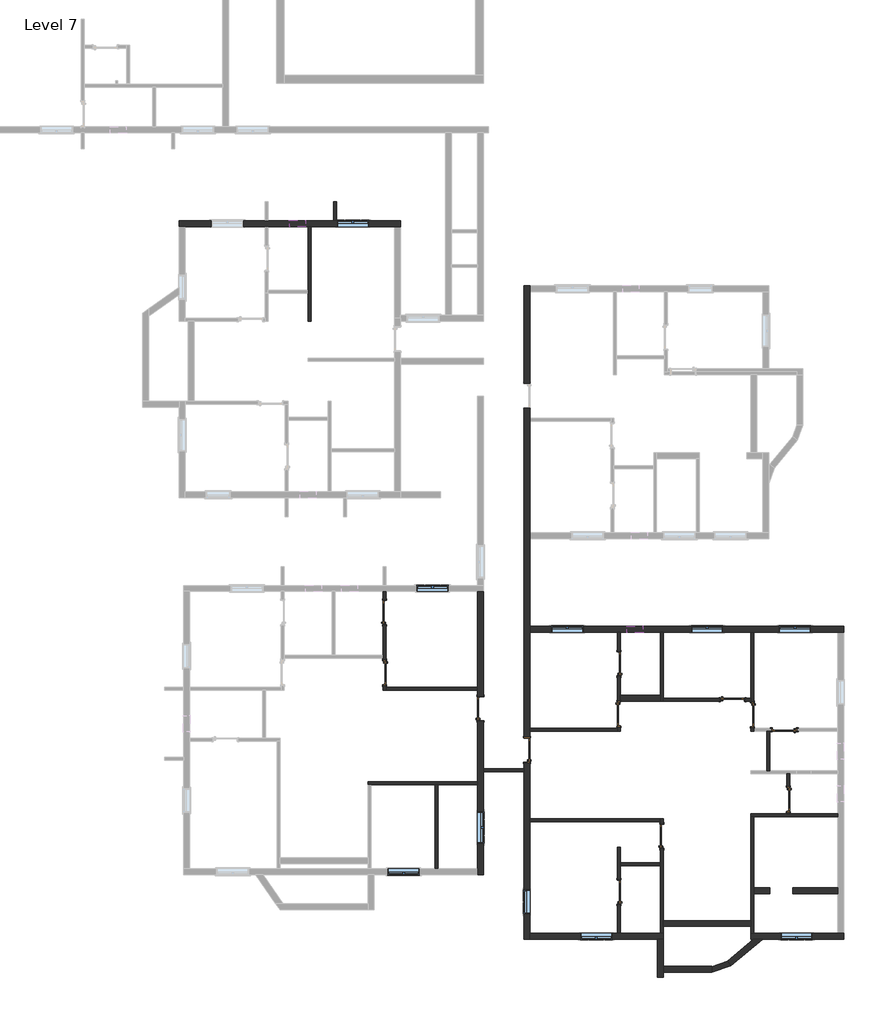
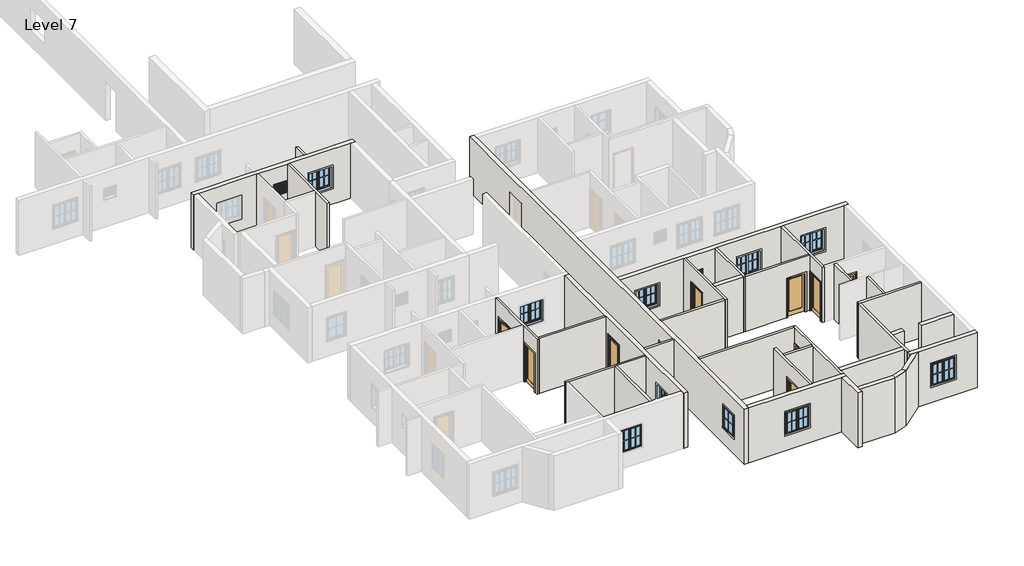
# One storey, part 2 of 7: 34 walls, 12 doors, 12 windows.
"""IFC4 building model written with IfcOpenShell, lengths in millimetres."""

from ifc_helpers import new_model, si_unit, frame, origin, place, context, project, spatial, polyline, circle_curve, outline, extrude, faceted_brep, transform, mapped, element, save
from ifc_brep_helpers import plane_surface, cylinder_surface, revolved_surface, advanced_brep
from components import door_3c6ab76a, door_a3feeac7, door_3b97b8e7, door_868ee8a9, window_272f20d6, window_casement_double_4_x_4_af3140d2, window_f2d8fef0

model = new_model("IFC4")

# Units and contexts
model_context = context("Model", 3, world=origin())
ifc_project = project(units=[si_unit("LENGTHUNIT", "METRE", prefix="MILLI")], contexts=[model_context])

# Site, building, storey
site = spatial("IfcSite", under=ifc_project)
building = spatial("IfcBuilding", under=site)
storey = spatial("IfcBuildingStorey", under=building, Name="Level 7", Elevation=9601.2)

# Doors
placement = place(None, origin())
door_shape = door_3c6ab76a(model_context)
element("IfcDoor", 1, ObjectType="Door-Interior-Single-1_Panel-Wood : 2'6\" x 7' door", at=placement, inside=storey, context=model_context, shape_type="MappedRepresentation", body=[
    mapped(door_shape, transform((13598.2490531, -20317.8247229, 9601.2), x_axis=(1.0, 0.0, 0.0), y_axis=(0.0, 1.0, 0.0), z_axis=(0.0, 0.0, 1.0))),
])
element("IfcDoor", 2, ObjectType="Door-Interior-Single-1_Panel-Wood : 2'6\" x 7' door", at=placement, inside=storey, context=model_context, shape_type="MappedRepresentation", body=[
    mapped(door_shape, transform((15579.4490531, -21467.1747229, 9601.2), x_axis=(-1.0, 0.0, 0.0), y_axis=(0.0, -1.0, 0.0), z_axis=(0.0, 0.0, 1.0))),
])
element("IfcDoor", 3, ObjectType="Door-Interior-Single-1_Panel-Wood : 2'6\" x 7' door", at=placement, inside=storey, context=model_context, shape_type="MappedRepresentation", body=[
    mapped(door_shape, transform((15735.0240531, -24130.9997229, 9601.2), x_axis=(0.0, -1.0, 0.0), y_axis=(1.0, 0.0, 0.0), z_axis=(0.0, 0.0, 1.0))),
])
element("IfcDoor", 4, ObjectType="Door-Interior-Single-1_Panel-Wood : 2'6\" x 7' door", at=placement, inside=storey, context=model_context, shape_type="MappedRepresentation", body=[
    mapped(door_shape, transform((285.4740531, -16985.9538828, 9601.2), x_axis=(0.0, 1.0, 0.0), y_axis=(-1.0, 0.0, 0.0), z_axis=(0.0, 0.0, 1.0))),
])
door_2_shape = door_a3feeac7(model_context)
element("IfcDoor", 5, ObjectType="Door-Interior-Single-1_Panel-Wood : 2'6\" x 7' door", at=placement, inside=storey, context=model_context, shape_type="MappedRepresentation", body=[
    mapped(door_2_shape, transform((9258.0240531, -18949.3997229, 9601.2), x_axis=(0.0, 1.0, 0.0), y_axis=(-1.0, 0.0, 0.0), z_axis=(0.0, 0.0, 1.0))),
])
element("IfcDoor", 6, ObjectType="Door-Interior-Single-1_Panel-Wood : 2'6\" x 7' door", at=placement, inside=storey, context=model_context, shape_type="MappedRepresentation", body=[
    mapped(door_2_shape, transform((9258.0240531, -27674.2997229, 9601.2), x_axis=(0.0, 1.0, 0.0), y_axis=(-1.0, 0.0, 0.0), z_axis=(0.0, 0.0, 1.0))),
])
element("IfcDoor", 7, ObjectType="Door-Interior-Single-1_Panel-Wood : 36\" x 84\"", at=placement, inside=storey, context=model_context, shape_type="MappedRepresentation", body=[
    mapped(door_shape, transform((14363.4240531, -20892.4997229, 9601.2), x_axis=(0.0, -1.0, 0.0), y_axis=(1.0, 0.0, 0.0), z_axis=(0.0, 0.0, 1.0))),
])
element("IfcDoor", 8, ObjectType="Door-Interior-Single-1_Panel-Wood : 36\" x 84\"", at=placement, inside=storey, context=model_context, shape_type="MappedRepresentation", body=[
    mapped(door_shape, transform((10889.9740531, -25540.6997229, 9601.2), x_axis=(0.0, 1.0, 0.0), y_axis=(-1.0, 0.0, 0.0), z_axis=(0.0, 0.0, 1.0))),
])
element("IfcDoor", 9, ObjectType="Door-Interior-Single-1_Panel-Wood : 36\" x 84\"", at=placement, inside=storey, context=model_context, shape_type="MappedRepresentation", body=[
    mapped(door_shape, transform((291.8240531, -19291.0038828, 9601.2), x_axis=(0.0, -1.0, 0.0), y_axis=(1.0, 0.0, 0.0), z_axis=(0.0, 0.0, 1.0))),
])
door_3_shape = door_3b97b8e7(model_context)
element("IfcDoor", 10, ObjectType="Door-Interior-Single-1_Panel-Wood : 36\" x 84\"", at=placement, inside=storey, context=model_context, shape_type="MappedRepresentation", body=[
    mapped(door_3_shape, transform((3962.1240531, -20662.6038828, 9601.2), x_axis=(0.0, 1.0, 0.0), y_axis=(-1.0, 0.0, 0.0), z_axis=(0.0, 0.0, 1.0))),
])
element("IfcDoor", 11, ObjectType="Door-Interior-Single-1_Panel-Wood : 36\" x 84\"", at=placement, inside=storey, context=model_context, shape_type="MappedRepresentation", body=[
    mapped(door_2_shape, transform((9251.6740531, -20863.9247229, 9601.2), x_axis=(0.0, -1.0, 0.0), y_axis=(1.0, 0.0, 0.0), z_axis=(0.0, 0.0, 1.0))),
])
door_4_shape = door_868ee8a9(model_context)
element("IfcDoor", 12, ObjectType="Door-Interior-Single-1_Panel-Wood : 36\" x 84\"", at=placement, inside=storey, context=model_context, shape_type="MappedRepresentation", body=[
    mapped(door_4_shape, transform((5733.7740531, -22245.3540434, 9601.2), x_axis=(0.0, 1.0, 0.0), y_axis=(-1.0, 0.0, 0.0), z_axis=(0.0, 0.0, 1.0))),
])

# Walls
element("IfcWall", 13, ObjectType="4.5\" wall", at=placement, inside=storey, context=model_context, shape_type="Brep", body=[
    faceted_brep([(-2524.4009469, -5860.7538828, 9601.2), (-2524.4009469, -2241.2538828, 9601.2), (-2524.4009469, -2241.2538828, 12649.2), (-2524.4009469, -5860.7538828, 12649.2), (-2638.7009469, -5860.7538828, 9601.2), (-2638.7009469, -5860.7538828, 12649.2), (-2638.7009469, -4793.9538828, 12649.2), (-2638.7009469, -4679.6538828, 12649.2), (-2638.7009469, -2241.2538828, 12649.2), (-2638.7009469, -2241.2538828, 9601.2), (-2638.7009469, -4679.6538828, 9601.2), (-2638.7009469, -4793.9538828, 9601.2)], [[[0, 1, 2, 3]], [[4, 5, 6, 7, 8, 9, 10, 11]], [[1, 0, 4, 11, 10, 9]], [[3, 2, 8, 7, 6, 5]], [[0, 3, 5, 4]], [[2, 1, 9, 8]]]),
])
element("IfcWall", 14, ObjectType="4.5\" wall", at=placement, inside=storey, context=model_context, shape_type="SweptSolid", body=[
    extrude(outline(polyline([(-1533.8009469, -1288.7538828), (-1533.8009469, -2012.6538828), (-1648.1009469, -2012.6538828), (-1648.1009469, -1288.7538828), (-1533.8009469, -1288.7538828)])), frame((0.0, 0.0, 9601.2), z_axis=(0.0, 0.0, 1.0), x_axis=(1.0, 0.0, 0.0)), (0.0, 0.0, 1.0), 3048.0),
])
element("IfcWall", 15, ObjectType="4.5\" wall", at=placement, inside=storey, context=model_context, shape_type="Brep", body=[
    faceted_brep([(345.7990531, -16185.8538828, 12649.2), (345.7990531, -19843.4538828, 12649.2), (345.7990531, -19957.7538828, 12649.2), (345.7990531, -19957.7538828, 9601.2), (345.7990531, -19843.4538828, 9601.2), (345.7990531, -19773.6038828, 9601.2), (345.7990531, -19773.6038828, 11760.2), (345.7990531, -18808.4038828, 11760.2), (345.7990531, -18808.4038828, 9601.2), (345.7990531, -17468.5538828, 9601.2), (345.7990531, -17468.5538828, 11760.2), (345.7990531, -16503.3538828, 11760.2), (345.7990531, -16503.3538828, 9601.2), (345.7990531, -16185.8538828, 9601.2), (231.4990531, -19957.7538828, 12649.2), (231.4990531, -18738.5538828, 12649.2), (231.4990531, -18624.2538828, 12649.2), (231.4990531, -16185.8538828, 12649.2), (231.4990531, -16185.8538828, 9601.2), (231.4990531, -16503.3538828, 9601.2), (231.4990531, -16503.3538828, 11760.2), (231.4990531, -17468.5538828, 11760.2), (231.4990531, -17468.5538828, 9601.2), (231.4990531, -18624.2538828, 9601.2), (231.4990531, -18738.5538828, 9601.2), (231.4990531, -18808.4038828, 9601.2), (231.4990531, -18808.4038828, 11760.2), (231.4990531, -19773.6038828, 11760.2), (231.4990531, -19773.6038828, 9601.2), (231.4990531, -19957.7538828, 9601.2)], [[[0, 1, 2, 3, 4, 5, 6, 7, 8, 9, 10, 11, 12, 13]], [[14, 15, 16, 17, 18, 19, 20, 21, 22, 23, 24, 25, 26, 27, 28, 29]], [[18, 13, 12, 19]], [[3, 29, 28, 5, 4]], [[22, 9, 8, 25, 24, 23]], [[2, 1, 0, 17, 16, 15, 14]], [[0, 13, 18, 17]], [[3, 2, 14, 29]], [[11, 20, 19, 12]], [[20, 11, 10, 21]], [[21, 10, 9, 22]], [[27, 6, 5, 28]], [[6, 27, 26, 7]], [[7, 26, 25, 8]]]),
])
element("IfcWall", 16, ObjectType="4.5\" wall", at=placement, inside=storey, context=model_context, shape_type="SweptSolid", body=[
    extrude(outline(polyline([(3850.9990531, -19957.7538828), (345.7990531, -19957.7538828), (345.7990531, -19843.4538828), (3850.9990531, -19843.4538828), (3850.9990531, -19957.7538828)])), frame((0.0, 0.0, 9601.2), z_axis=(0.0, 0.0, 1.0), x_axis=(1.0, 0.0, 0.0)), (0.0, 0.0, 1.0), 3048.0),
])
element("IfcWall", 17, ObjectType="4.5\" wall", at=placement, inside=storey, context=model_context, shape_type="Brep", body=[
    faceted_brep([(3850.9990531, -23462.9538828, 9601.2), (-340.0009469, -23462.9538828, 9601.2), (-340.0009469, -23462.9538828, 12649.2), (3850.9990531, -23462.9538828, 12649.2), (3850.9990531, -23577.2538828, 9601.2), (3850.9990531, -23577.2538828, 12649.2), (2326.9990531, -23577.2538828, 12649.2), (2212.6990531, -23577.2538828, 12649.2), (-225.7009469, -23577.2538828, 12649.2), (-340.0009469, -23577.2538828, 12649.2), (-340.0009469, -23577.2538828, 9601.2), (-225.7009469, -23577.2538828, 9601.2), (2212.6990531, -23577.2538828, 9601.2), (2326.9990531, -23577.2538828, 9601.2)], [[[0, 1, 2, 3]], [[4, 5, 6, 7, 8, 9, 10, 11, 12, 13]], [[1, 0, 4, 13, 12, 11, 10]], [[3, 2, 9, 8, 7, 6, 5]], [[0, 3, 5, 4]], [[2, 1, 10, 9]]]),
])
element("IfcWall", 18, ObjectType="4.5\" wall", at=placement, inside=storey, context=model_context, shape_type="SweptSolid", body=[
    extrude(outline(polyline([(2326.9990531, -23577.2538828), (2326.9990531, -26777.6538828), (2212.6990531, -26777.6538828), (2212.6990531, -23577.2538828), (2326.9990531, -23577.2538828)])), frame((0.0, 0.0, 9601.2), z_axis=(0.0, 0.0, 1.0), x_axis=(1.0, 0.0, 0.0)), (0.0, 0.0, 1.0), 3048.0),
])
element("IfcWall", 19, ObjectType="4.5\" wall", at=placement, inside=storey, context=model_context, shape_type="Brep", body=[
    faceted_brep([(10835.9990531, -17749.2497229, 9601.2), (10835.9990531, -20149.5497229, 9601.2), (10835.9990531, -20378.1497229, 9601.2), (10835.9990531, -20378.1497229, 12649.2), (10835.9990531, -20149.5497229, 12649.2), (10835.9990531, -17749.2497229, 12649.2), (10950.2990531, -17749.2497229, 9601.2), (10950.2990531, -17749.2497229, 12649.2), (10950.2990531, -20263.8497229, 12649.2), (10950.2990531, -20378.1497229, 12649.2), (10950.2990531, -20378.1497229, 9601.2), (10950.2990531, -20263.8497229, 9601.2)], [[[0, 1, 2, 3, 4, 5]], [[6, 7, 8, 9, 10, 11]], [[2, 1, 0, 6, 11, 10]], [[5, 4, 3, 9, 8, 7]], [[0, 5, 7, 6]], [[3, 2, 10, 9]]]),
])
element("IfcWall", 20, ObjectType="4.5\" wall", at=placement, inside=storey, context=model_context, shape_type="Brep", body=[
    faceted_brep([(9311.9990531, -17749.2497229, 12649.2), (9311.9990531, -20149.5497229, 12649.2), (9311.9990531, -20378.1497229, 12649.2), (9311.9990531, -21521.1497229, 12649.2), (9311.9990531, -21521.1497229, 9601.2), (9311.9990531, -21346.5247229, 9601.2), (9311.9990531, -21346.5247229, 11760.2), (9311.9990531, -20381.3247229, 11760.2), (9311.9990531, -20381.3247229, 9601.2), (9311.9990531, -20378.1497229, 9601.2), (9311.9990531, -20149.5497229, 9601.2), (9311.9990531, -19431.9997229, 9601.2), (9311.9990531, -19431.9997229, 11760.2), (9311.9990531, -18466.7997229, 11760.2), (9311.9990531, -18466.7997229, 9601.2), (9311.9990531, -17749.2497229, 9601.2), (9197.6990531, -21521.1497229, 12649.2), (9197.6990531, -21406.8497229, 12649.2), (9197.6990531, -17749.2497229, 12649.2), (9197.6990531, -17749.2497229, 9601.2), (9197.6990531, -18466.7997229, 9601.2), (9197.6990531, -18466.7997229, 11760.2), (9197.6990531, -19431.9997229, 11760.2), (9197.6990531, -19431.9997229, 9601.2), (9197.6990531, -20381.3247229, 9601.2), (9197.6990531, -20381.3247229, 11760.2), (9197.6990531, -21346.5247229, 11760.2), (9197.6990531, -21346.5247229, 9601.2), (9197.6990531, -21406.8497229, 9601.2), (9197.6990531, -21521.1497229, 9601.2)], [[[0, 1, 2, 3, 4, 5, 6, 7, 8, 9, 10, 11, 12, 13, 14, 15]], [[16, 17, 18, 19, 20, 21, 22, 23, 24, 25, 26, 27, 28, 29]], [[19, 15, 14, 20]], [[4, 29, 28, 27, 5]], [[8, 24, 23, 11, 10, 9]], [[3, 2, 1, 0, 18, 17, 16]], [[0, 15, 19, 18]], [[4, 3, 16, 29]], [[26, 6, 5, 27]], [[6, 26, 25, 7]], [[7, 25, 24, 8]], [[13, 21, 20, 14]], [[21, 13, 12, 22]], [[22, 12, 11, 23]]]),
])
element("IfcWall", 21, ObjectType="4.5\" wall", at=placement, inside=storey, context=model_context, shape_type="SweptSolid", body=[
    extrude(outline(polyline([(5844.8990531, -21406.8497229), (9197.6990531, -21406.8497229), (9197.6990531, -21521.1497229), (5844.8990531, -21521.1497229), (5844.8990531, -21406.8497229)])), frame((0.0, 0.0, 9601.2), z_axis=(0.0, 0.0, 1.0), x_axis=(1.0, 0.0, 0.0)), (0.0, 0.0, 1.0), 3048.0),
])
element("IfcWall", 22, ObjectType="4.5\" wall", at=placement, inside=storey, context=model_context, shape_type="Brep", body=[
    faceted_brep([(14303.0990531, -21521.1497229, 12649.2), (14303.0990531, -20378.1497229, 12649.2), (14303.0990531, -20263.8497229, 12649.2), (14303.0990531, -17749.2497229, 12649.2), (14303.0990531, -17749.2497229, 9601.2), (14303.0990531, -20263.8497229, 9601.2), (14303.0990531, -20378.1497229, 9601.2), (14303.0990531, -20409.8997229, 9601.2), (14303.0990531, -20409.8997229, 11760.2), (14303.0990531, -21375.0997229, 11760.2), (14303.0990531, -21375.0997229, 9601.2), (14303.0990531, -21521.1497229, 9601.2), (14417.3990531, -17749.2497229, 12649.2), (14417.3990531, -21406.8497229, 12649.2), (14417.3990531, -21521.1497229, 12649.2), (14417.3990531, -21521.1497229, 9601.2), (14417.3990531, -21406.8497229, 9601.2), (14417.3990531, -21375.0997229, 9601.2), (14417.3990531, -21375.0997229, 11760.2), (14417.3990531, -20409.8997229, 11760.2), (14417.3990531, -20409.8997229, 9601.2), (14417.3990531, -17749.2497229, 9601.2)], [[[0, 1, 2, 3, 4, 5, 6, 7, 8, 9, 10, 11]], [[12, 13, 14, 15, 16, 17, 18, 19, 20, 21]], [[4, 21, 20, 7, 6, 5]], [[15, 11, 10, 17, 16]], [[3, 2, 1, 0, 14, 13, 12]], [[4, 3, 12, 21]], [[0, 11, 15, 14]], [[9, 18, 17, 10]], [[18, 9, 8, 19]], [[19, 8, 7, 20]]]),
])
element("IfcWall", 23, ObjectType="4.5\" wall", at=placement, inside=storey, context=model_context, shape_type="Brep", body=[
    faceted_brep([(14303.0990531, -24797.7497229, 9601.2), (14417.3990531, -24797.7497229, 9601.2), (17617.7990531, -24797.7497229, 9601.2), (17617.7990531, -24797.7497229, 12649.2), (14417.3990531, -24797.7497229, 12649.2), (14303.0990531, -24797.7497229, 12649.2), (14303.0990531, -24683.4497229, 9601.2), (14303.0990531, -24683.4497229, 12649.2), (15674.6990531, -24683.4497229, 12649.2), (15788.9990531, -24683.4497229, 12649.2), (17617.7990531, -24683.4497229, 12649.2), (17617.7990531, -24683.4497229, 9601.2), (15788.9990531, -24683.4497229, 9601.2), (15674.6990531, -24683.4497229, 9601.2)], [[[0, 1, 2, 3, 4, 5]], [[6, 7, 8, 9, 10, 11, 12, 13]], [[2, 1, 0, 6, 13, 12, 11]], [[5, 4, 3, 10, 9, 8, 7]], [[3, 2, 11, 10]], [[0, 5, 7, 6]]]),
])
element("IfcWall", 24, ObjectType="4.5\" wall", at=placement, inside=storey, context=model_context, shape_type="Brep", body=[
    faceted_brep([(14417.3990531, -29255.4497229, 9601.2), (14417.3990531, -27731.4497229, 9601.2), (14417.3990531, -27502.8497229, 9601.2), (14417.3990531, -24797.7497229, 9601.2), (14417.3990531, -24797.7497229, 12649.2), (14417.3990531, -27502.8497229, 12649.2), (14417.3990531, -27731.4497229, 12649.2), (14417.3990531, -29255.4497229, 12649.2), (14303.0990531, -29255.4497229, 9601.2), (14303.0990531, -29255.4497229, 12649.2), (14303.0990531, -28988.7497229, 12649.2), (14303.0990531, -28760.1497229, 12649.2), (14303.0990531, -24797.7497229, 12649.2), (14303.0990531, -24797.7497229, 9601.2), (14303.0990531, -28760.1497229, 9601.2), (14303.0990531, -28988.7497229, 9601.2)], [[[0, 1, 2, 3, 4, 5, 6, 7]], [[8, 9, 10, 11, 12, 13, 14, 15]], [[3, 2, 1, 0, 8, 15, 14, 13]], [[7, 6, 5, 4, 12, 11, 10, 9]], [[4, 3, 13, 12]], [[0, 7, 9, 8]]]),
])
element("IfcWall", 25, ObjectType="4.5\" wall", at=placement, inside=storey, context=model_context, shape_type="SweptSolid", body=[
    extrude(outline(polyline([(12649.2, 14303.0990531), (12649.2, 10950.2990531), (9601.2, 10950.2990531), (9601.2, 13115.6490531), (11760.2, 13115.6490531), (11760.2, 14080.8490531), (9601.2, 14080.8490531), (9601.2, 14303.0990531), (12649.2, 14303.0990531)])), frame((0.0, -20378.1497229, 0.0), z_axis=(0.0, 1.0, 0.0), x_axis=(0.0, 0.0, 1.0)), (0.0, 0.0, 1.0), 114.3),
])
element("IfcWall", 26, ObjectType="4.5\" wall", at=placement, inside=storey, context=model_context, shape_type="SweptSolid", body=[
    extrude(outline(polyline([(14912.6990531, -23045.1497229), (14912.6990531, -21521.1497229), (15026.9990531, -21521.1497229), (15026.9990531, -23045.1497229), (14912.6990531, -23045.1497229)])), frame((0.0, 0.0, 9601.2), z_axis=(0.0, 0.0, 1.0), x_axis=(1.0, 0.0, 0.0)), (0.0, 0.0, 1.0), 3048.0),
])
element("IfcWall", 27, ObjectType="4.5\" wall", at=placement, inside=storey, context=model_context, shape_type="Brep", body=[
    faceted_brep([(10835.9990531, -29255.4497229, 12649.2), (10835.9990531, -26664.6497229, 12649.2), (10835.9990531, -26550.3497229, 12649.2), (10835.9990531, -24988.2497229, 12649.2), (10835.9990531, -24873.9497229, 12649.2), (10835.9990531, -24873.9497229, 9601.2), (10835.9990531, -24988.2497229, 9601.2), (10835.9990531, -25058.0997229, 9601.2), (10835.9990531, -25058.0997229, 11760.2), (10835.9990531, -26023.2997229, 11760.2), (10835.9990531, -26023.2997229, 9601.2), (10835.9990531, -26550.3497229, 9601.2), (10835.9990531, -26664.6497229, 9601.2), (10835.9990531, -29255.4497229, 9601.2), (10950.2990531, -24873.9497229, 12649.2), (10950.2990531, -28760.1497229, 12649.2), (10950.2990531, -28988.7497229, 12649.2), (10950.2990531, -29255.4497229, 12649.2), (10950.2990531, -29255.4497229, 9601.2), (10950.2990531, -28988.7497229, 9601.2), (10950.2990531, -28760.1497229, 9601.2), (10950.2990531, -26023.2997229, 9601.2), (10950.2990531, -26023.2997229, 11760.2), (10950.2990531, -25058.0997229, 11760.2), (10950.2990531, -25058.0997229, 9601.2), (10950.2990531, -24873.9497229, 9601.2)], [[[0, 1, 2, 3, 4, 5, 6, 7, 8, 9, 10, 11, 12, 13]], [[14, 15, 16, 17, 18, 19, 20, 21, 22, 23, 24, 25]], [[18, 13, 12, 11, 10, 21, 20, 19]], [[5, 25, 24, 7, 6]], [[4, 3, 2, 1, 0, 17, 16, 15, 14]], [[0, 13, 18, 17]], [[5, 4, 14, 25]], [[23, 8, 7, 24]], [[8, 23, 22, 9]], [[9, 22, 21, 10]]]),
])
element("IfcWall", 28, ObjectType="4.5\" wall", at=placement, inside=storey, context=model_context, shape_type="SweptSolid", body=[
    extrude(outline(polyline([(10835.9990531, -24988.2497229), (5844.8990531, -24988.2497229), (5844.8990531, -24873.9497229), (10835.9990531, -24873.9497229), (10835.9990531, -24988.2497229)])), frame((0.0, 0.0, 9601.2), z_axis=(0.0, 0.0, 1.0), x_axis=(1.0, 0.0, 0.0)), (0.0, 0.0, 1.0), 3048.0),
])
element("IfcWall", 29, ObjectType="4.5\" wall", at=placement, inside=storey, context=model_context, shape_type="SweptSolid", body=[
    extrude(outline(polyline([(-24683.4497229, 12649.2), (-23159.4497229, 12649.2), (-23159.4497229, 9601.2), (-23648.3997229, 9601.2), (-23648.3997229, 11760.2), (-24613.5997229, 11760.2), (-24613.5997229, 9601.2), (-24683.4497229, 9601.2), (-24683.4497229, 12649.2)])), frame((15674.6990531, 0.0, 0.0), z_axis=(1.0, 0.0, 0.0), x_axis=(0.0, 1.0, 0.0)), (0.0, 0.0, 1.0), 114.3),
])
element("IfcWall", 30, ObjectType="4.5\" wall", at=placement, inside=storey, context=model_context, shape_type="SweptSolid", body=[
    extrude(outline(polyline([(10835.9990531, -26664.6497229), (9311.9990531, -26664.6497229), (9311.9990531, -26550.3497229), (10835.9990531, -26550.3497229), (10835.9990531, -26664.6497229)])), frame((0.0, 0.0, 9601.2), z_axis=(0.0, 0.0, 1.0), x_axis=(1.0, 0.0, 0.0)), (0.0, 0.0, 1.0), 3048.0),
])
element("IfcWall", 31, ObjectType="4.5\" wall", at=placement, inside=storey, context=model_context, shape_type="Brep", body=[
    faceted_brep([(9311.9990531, -25953.4497229, 9601.2), (9311.9990531, -25953.4497229, 12649.2), (9311.9990531, -26550.3497229, 12649.2), (9311.9990531, -26664.6497229, 12649.2), (9311.9990531, -29255.4497229, 12649.2), (9311.9990531, -29255.4497229, 9601.2), (9311.9990531, -28156.8997229, 9601.2), (9311.9990531, -28156.8997229, 11760.2), (9311.9990531, -27191.6997229, 11760.2), (9311.9990531, -27191.6997229, 9601.2), (9311.9990531, -26664.6497229, 9601.2), (9311.9990531, -26550.3497229, 9601.2), (9197.6990531, -25953.4497229, 12649.2), (9197.6990531, -25953.4497229, 9601.2), (9197.6990531, -27191.6997229, 9601.2), (9197.6990531, -27191.6997229, 11760.2), (9197.6990531, -28156.8997229, 11760.2), (9197.6990531, -28156.8997229, 9601.2), (9197.6990531, -29255.4497229, 9601.2), (9197.6990531, -29255.4497229, 12649.2)], [[[0, 1, 2, 3, 4, 5, 6, 7, 8, 9, 10, 11]], [[12, 13, 14, 15, 16, 17, 18, 19]], [[13, 0, 11, 10, 9, 14]], [[5, 18, 17, 6]], [[1, 0, 13, 12]], [[4, 3, 2, 1, 12, 19]], [[5, 4, 19, 18]], [[8, 15, 14, 9]], [[15, 8, 7, 16]], [[16, 7, 6, 17]]]),
])
element("IfcWall", 32, ObjectType="4.5\" wall", at=placement, inside=storey, context=model_context, shape_type="SweptSolid", body=[
    extrude(outline(polyline([(4079.5990531, -22969.5583639), (5616.2990531, -22969.5583639), (5616.2990531, -23083.8583639), (4079.5990531, -23083.8583639), (4079.5990531, -22969.5583639)])), frame((0.0, 0.0, 9601.2), z_axis=(0.0, 0.0, 1.0), x_axis=(1.0, 0.0, 0.0)), (0.0, 0.0, 1.0), 3048.0),
])
element("IfcWall", 33, ObjectType="9\"", at=placement, inside=storey, context=model_context, shape_type="Brep", body=[
    faceted_brep([(904.5990531, -2012.6538828, 9601.2), (-1533.8009469, -2012.6538828, 9601.2), (-1648.1009469, -2012.6538828, 9601.2), (-4162.7009469, -2012.6538828, 9601.2), (-4277.0009469, -2012.6538828, 9601.2), (-7553.6009469, -2012.6538828, 9601.2), (-7553.6009469, -2012.6538828, 12649.2), (-4277.0009469, -2012.6538828, 12649.2), (-4162.7009469, -2012.6538828, 12649.2), (-1648.1009469, -2012.6538828, 12649.2), (-1533.8009469, -2012.6538828, 12649.2), (904.5990531, -2012.6538828, 12649.2), (-2733.9509469, -2012.6538828, 11734.8), (-3343.5509469, -2012.6538828, 11734.8), (-3343.5509469, -2012.6538828, 11125.2), (-2733.9509469, -2012.6538828, 11125.2), (-5108.8509469, -2012.6538828, 11734.8), (-6328.0509469, -2012.6538828, 11734.8), (-6328.0509469, -2012.6538828, 10515.6), (-5108.8509469, -2012.6538828, 10515.6), (-308.2509469, -2012.6538828, 11734.8), (-1527.4509469, -2012.6538828, 11734.8), (-1527.4509469, -2012.6538828, 10515.6), (-308.2509469, -2012.6538828, 10515.6), (904.5990531, -2241.2538828, 9601.2), (904.5990531, -2241.2538828, 12649.2), (675.9990531, -2241.2538828, 12649.2), (-2524.4009469, -2241.2538828, 12649.2), (-2638.7009469, -2241.2538828, 12649.2), (-4162.7009469, -2241.2538828, 12649.2), (-4277.0009469, -2241.2538828, 12649.2), (-7325.0009469, -2241.2538828, 12649.2), (-7553.6009469, -2241.2538828, 12649.2), (-7553.6009469, -2241.2538828, 9601.2), (-7325.0009469, -2241.2538828, 9601.2), (-4277.0009469, -2241.2538828, 9601.2), (-4162.7009469, -2241.2538828, 9601.2), (-2638.7009469, -2241.2538828, 9601.2), (-2524.4009469, -2241.2538828, 9601.2), (675.9990531, -2241.2538828, 9601.2), (-2733.9509469, -2241.2538828, 11734.8), (-2733.9509469, -2241.2538828, 11125.2), (-3343.5509469, -2241.2538828, 11125.2), (-3343.5509469, -2241.2538828, 11734.8), (-5108.8509469, -2241.2538828, 11734.8), (-5108.8509469, -2241.2538828, 10515.6), (-6328.0509469, -2241.2538828, 10515.6), (-6328.0509469, -2241.2538828, 11734.8), (-308.2509469, -2241.2538828, 11734.8), (-308.2509469, -2241.2538828, 10515.6), (-1527.4509469, -2241.2538828, 10515.6), (-1527.4509469, -2241.2538828, 11734.8)], [[[0, 1, 2, 3, 4, 5, 6, 7, 8, 9, 10, 11], [12, 13, 14, 15], [16, 17, 18, 19], [20, 21, 22, 23]], [[24, 25, 26, 27, 28, 29, 30, 31, 32, 33, 34, 35, 36, 37, 38, 39], [40, 41, 42, 43], [44, 45, 46, 47], [48, 49, 50, 51]], [[5, 4, 3, 2, 1, 0, 24, 39, 38, 37, 36, 35, 34, 33]], [[11, 10, 9, 8, 7, 6, 32, 31, 30, 29, 28, 27, 26, 25]], [[0, 11, 25, 24]], [[6, 5, 33, 32]], [[41, 40, 12, 15]], [[42, 41, 15, 14]], [[43, 42, 14, 13]], [[40, 43, 13, 12]], [[45, 44, 16, 19]], [[46, 45, 19, 18]], [[47, 46, 18, 17]], [[44, 47, 17, 16]], [[49, 48, 20, 23]], [[50, 49, 23, 22]], [[51, 50, 22, 21]], [[48, 51, 21, 20]]]),
])
element("IfcWall", 34, ObjectType="9\"", at=placement, inside=storey, context=model_context, shape_type="Brep", body=[
    faceted_brep([(4079.5990531, -16185.8538828, 12649.2), (4079.5990531, -22969.5583639, 12649.2), (4079.5990531, -23083.8583639, 12649.2), (4079.5990531, -27006.2538828, 12649.2), (4079.5990531, -27006.2538828, 9601.2), (4079.5990531, -23083.8583639, 9601.2), (4079.5990531, -22969.5583639, 9601.2), (4079.5990531, -21145.2038828, 9601.2), (4079.5990531, -21145.2038828, 11760.2), (4079.5990531, -20180.0038828, 11760.2), (4079.5990531, -20180.0038828, 9601.2), (4079.5990531, -16185.8538828, 9601.2), (4079.5990531, -25815.6288828, 11734.8), (4079.5990531, -24596.4288828, 11734.8), (4079.5990531, -24596.4288828, 10515.6), (4079.5990531, -25815.6288828, 10515.6), (3850.9990531, -27006.2538828, 12649.2), (3850.9990531, -26777.6538828, 12649.2), (3850.9990531, -23577.2538828, 12649.2), (3850.9990531, -23462.9538828, 12649.2), (3850.9990531, -19957.7538828, 12649.2), (3850.9990531, -19843.4538828, 12649.2), (3850.9990531, -16185.8538828, 12649.2), (3850.9990531, -16185.8538828, 9601.2), (3850.9990531, -19843.4538828, 9601.2), (3850.9990531, -19957.7538828, 9601.2), (3850.9990531, -20180.0038828, 9601.2), (3850.9990531, -20180.0038828, 11760.2), (3850.9990531, -21145.2038828, 11760.2), (3850.9990531, -21145.2038828, 9601.2), (3850.9990531, -23462.9538828, 9601.2), (3850.9990531, -23577.2538828, 9601.2), (3850.9990531, -26777.6538828, 9601.2), (3850.9990531, -27006.2538828, 9601.2), (3850.9990531, -25815.6288828, 11734.8), (3850.9990531, -25815.6288828, 10515.6), (3850.9990531, -24596.4288828, 10515.6), (3850.9990531, -24596.4288828, 11734.8)], [[[0, 1, 2, 3, 4, 5, 6, 7, 8, 9, 10, 11], [12, 13, 14, 15]], [[16, 17, 18, 19, 20, 21, 22, 23, 24, 25, 26, 27, 28, 29, 30, 31, 32, 33], [34, 35, 36, 37]], [[4, 33, 32, 31, 30, 29, 7, 6, 5]], [[23, 11, 10, 26, 25, 24]], [[3, 2, 1, 0, 22, 21, 20, 19, 18, 17, 16]], [[4, 3, 16, 33]], [[0, 11, 23, 22]], [[9, 27, 26, 10]], [[27, 9, 8, 28]], [[28, 8, 7, 29]], [[35, 34, 12, 15]], [[36, 35, 15, 14]], [[37, 36, 14, 13]], [[34, 37, 13, 12]]]),
])
element("IfcWall", 35, ObjectType="9\"", at=placement, inside=storey, context=model_context, shape_type="Brep", body=[
    faceted_brep([(5844.8990531, -17749.2497229, 9601.2), (9197.6990531, -17749.2497229, 9601.2), (9311.9990531, -17749.2497229, 9601.2), (10835.9990531, -17749.2497229, 9601.2), (10950.2990531, -17749.2497229, 9601.2), (14303.0990531, -17749.2497229, 9601.2), (14417.3990531, -17749.2497229, 9601.2), (17617.7990531, -17749.2497229, 9601.2), (17846.3990531, -17749.2497229, 9601.2), (17846.3990531, -17749.2497229, 12649.2), (17617.7990531, -17749.2497229, 12649.2), (14417.3990531, -17749.2497229, 12649.2), (14303.0990531, -17749.2497229, 12649.2), (10950.2990531, -17749.2497229, 12649.2), (10835.9990531, -17749.2497229, 12649.2), (9311.9990531, -17749.2497229, 12649.2), (9197.6990531, -17749.2497229, 12649.2), (5844.8990531, -17749.2497229, 12649.2), (10169.2490531, -17749.2497229, 11734.8), (10169.2490531, -17749.2497229, 11125.2), (9559.6490531, -17749.2497229, 11125.2), (9559.6490531, -17749.2497229, 11734.8), (7889.5990531, -17749.2497229, 11734.8), (7889.5990531, -17749.2497229, 10515.6), (6670.3990531, -17749.2497229, 10515.6), (6670.3990531, -17749.2497229, 11734.8), (13236.2990531, -17749.2497229, 11734.8), (13236.2990531, -17749.2497229, 10515.6), (12017.0990531, -17749.2497229, 10515.6), (12017.0990531, -17749.2497229, 11734.8), (16595.4490531, -17749.2497229, 11734.8), (16595.4490531, -17749.2497229, 10515.6), (15376.2490531, -17749.2497229, 10515.6), (15376.2490531, -17749.2497229, 11734.8), (5844.8990531, -17520.6497229, 9601.2), (5844.8990531, -17520.6497229, 12649.2), (17846.3990531, -17520.6497229, 12649.2), (17846.3990531, -17520.6497229, 9601.2), (10169.2490531, -17520.6497229, 11734.8), (9559.6490531, -17520.6497229, 11734.8), (9559.6490531, -17520.6497229, 11125.2), (10169.2490531, -17520.6497229, 11125.2), (7889.5990531, -17520.6497229, 11734.8), (6670.3990531, -17520.6497229, 11734.8), (6670.3990531, -17520.6497229, 10515.6), (7889.5990531, -17520.6497229, 10515.6), (13236.2990531, -17520.6497229, 11734.8), (12017.0990531, -17520.6497229, 11734.8), (12017.0990531, -17520.6497229, 10515.6), (13236.2990531, -17520.6497229, 10515.6), (16595.4490531, -17520.6497229, 11734.8), (15376.2490531, -17520.6497229, 11734.8), (15376.2490531, -17520.6497229, 10515.6), (16595.4490531, -17520.6497229, 10515.6)], [[[0, 1, 2, 3, 4, 5, 6, 7, 8, 9, 10, 11, 12, 13, 14, 15, 16, 17], [18, 19, 20, 21], [22, 23, 24, 25], [26, 27, 28, 29], [30, 31, 32, 33]], [[34, 35, 36, 37], [38, 39, 40, 41], [42, 43, 44, 45], [46, 47, 48, 49], [50, 51, 52, 53]], [[8, 7, 6, 5, 4, 3, 2, 1, 0, 34, 37]], [[17, 16, 15, 14, 13, 12, 11, 10, 9, 36, 35]], [[0, 17, 35, 34]], [[9, 8, 37, 36]], [[19, 18, 38, 41]], [[20, 19, 41, 40]], [[21, 20, 40, 39]], [[18, 21, 39, 38]], [[23, 22, 42, 45]], [[24, 23, 45, 44]], [[25, 24, 44, 43]], [[22, 25, 43, 42]], [[27, 26, 46, 49]], [[28, 27, 49, 48]], [[29, 28, 48, 47]], [[26, 29, 47, 46]], [[31, 30, 50, 53]], [[32, 31, 53, 52]], [[33, 32, 52, 51]], [[30, 33, 51, 50]]]),
])
element("IfcWall", 36, ObjectType="9\"", at=placement, inside=storey, context=model_context, shape_type="Brep", body=[
    faceted_brep([(5844.8990531, -4503.1497229, 12649.2), (5844.8990531, -4731.7497229, 12649.2), (5844.8990531, -9557.7497229, 12649.2), (5844.8990531, -9672.0497229, 12649.2), (5844.8990531, -13939.2497229, 12649.2), (5844.8990531, -14167.8497229, 12649.2), (5844.8990531, -17520.6497229, 12649.2), (5844.8990531, -17749.2497229, 12649.2), (5844.8990531, -21406.8497229, 12649.2), (5844.8990531, -21521.1497229, 12649.2), (5844.8990531, -24873.9497229, 12649.2), (5844.8990531, -24988.2497229, 12649.2), (5844.8990531, -29255.4497229, 12649.2), (5844.8990531, -29484.0497229, 12649.2), (5844.8990531, -29484.0497229, 9601.2), (5844.8990531, -29255.4497229, 9601.2), (5844.8990531, -24988.2497229, 9601.2), (5844.8990531, -24873.9497229, 9601.2), (5844.8990531, -22727.9540434, 9601.2), (5844.8990531, -22727.9540434, 11760.2), (5844.8990531, -21762.7540434, 11760.2), (5844.8990531, -21762.7540434, 9601.2), (5844.8990531, -21521.1497229, 9601.2), (5844.8990531, -21406.8497229, 9601.2), (5844.8990531, -17749.2497229, 9601.2), (5844.8990531, -17520.6497229, 9601.2), (5844.8990531, -14167.8497229, 9601.2), (5844.8990531, -13939.2497229, 9601.2), (5844.8990531, -9672.0497229, 9601.2), (5844.8990531, -9557.7497229, 9601.2), (5844.8990531, -9183.0997229, 9601.2), (5844.8990531, -9183.0997229, 11760.2), (5844.8990531, -8217.8997229, 11760.2), (5844.8990531, -8217.8997229, 9601.2), (5844.8990531, -4731.7497229, 9601.2), (5844.8990531, -4503.1497229, 9601.2), (5844.8990531, -27591.7497229, 11734.8), (5844.8990531, -27591.7497229, 10515.6), (5844.8990531, -28506.1497229, 10515.6), (5844.8990531, -28506.1497229, 11734.8), (5616.2990531, -29484.0497229, 12649.2), (5616.2990531, -23083.8583639, 12649.2), (5616.2990531, -22969.5583639, 12649.2), (5616.2990531, -4503.1497229, 12649.2), (5616.2990531, -4503.1497229, 9601.2), (5616.2990531, -8217.8997229, 9601.2), (5616.2990531, -8217.8997229, 11760.2), (5616.2990531, -9183.0997229, 11760.2), (5616.2990531, -9183.0997229, 9601.2), (5616.2990531, -21762.7540434, 9601.2), (5616.2990531, -21762.7540434, 11760.2), (5616.2990531, -22727.9540434, 11760.2), (5616.2990531, -22727.9540434, 9601.2), (5616.2990531, -22969.5583639, 9601.2), (5616.2990531, -23083.8583639, 9601.2), (5616.2990531, -29484.0497229, 9601.2), (5616.2990531, -27591.7497229, 11734.8), (5616.2990531, -28506.1497229, 11734.8), (5616.2990531, -28506.1497229, 10515.6), (5616.2990531, -27591.7497229, 10515.6)], [[[0, 1, 2, 3, 4, 5, 6, 7, 8, 9, 10, 11, 12, 13, 14, 15, 16, 17, 18, 19, 20, 21, 22, 23, 24, 25, 26, 27, 28, 29, 30, 31, 32, 33, 34, 35], [36, 37, 38, 39]], [[40, 41, 42, 43, 44, 45, 46, 47, 48, 49, 50, 51, 52, 53, 54, 55], [56, 57, 58, 59]], [[14, 55, 54, 53, 52, 18, 17, 16, 15]], [[44, 35, 34, 33, 45]], [[48, 30, 29, 28, 27, 26, 25, 24, 23, 22, 21, 49]], [[13, 12, 11, 10, 9, 8, 7, 6, 5, 4, 3, 2, 1, 0, 43, 42, 41, 40]], [[14, 13, 40, 55]], [[0, 35, 44, 43]], [[47, 31, 30, 48]], [[31, 47, 46, 32]], [[32, 46, 45, 33]], [[20, 50, 49, 21]], [[50, 20, 19, 51]], [[51, 19, 18, 52]], [[37, 36, 56, 59]], [[38, 37, 59, 58]], [[39, 38, 58, 57]], [[36, 39, 57, 56]]]),
])
element("IfcWall", 37, ObjectType="9\"", at=placement, inside=storey, context=model_context, shape_type="Brep", body=[
    faceted_brep([(5844.8990531, -29484.0497229, 9601.2), (10721.6990531, -29484.0497229, 9601.2), (10950.2990531, -29484.0497229, 9601.2), (10950.2990531, -29484.0497229, 12649.2), (10721.6990531, -29484.0497229, 12649.2), (5844.8990531, -29484.0497229, 12649.2), (7781.6490531, -29484.0497229, 11734.8), (9000.8490531, -29484.0497229, 11734.8), (9000.8490531, -29484.0497229, 10515.6), (7781.6490531, -29484.0497229, 10515.6), (5844.8990531, -29255.4497229, 9601.2), (5844.8990531, -29255.4497229, 12649.2), (9197.6990531, -29255.4497229, 12649.2), (9311.9990531, -29255.4497229, 12649.2), (10835.9990531, -29255.4497229, 12649.2), (10950.2990531, -29255.4497229, 12649.2), (10950.2990531, -29255.4497229, 9601.2), (10835.9990531, -29255.4497229, 9601.2), (9311.9990531, -29255.4497229, 9601.2), (9197.6990531, -29255.4497229, 9601.2), (7781.6490531, -29255.4497229, 11734.8), (7781.6490531, -29255.4497229, 10515.6), (9000.8490531, -29255.4497229, 10515.6), (9000.8490531, -29255.4497229, 11734.8)], [[[0, 1, 2, 3, 4, 5], [6, 7, 8, 9]], [[10, 11, 12, 13, 14, 15, 16, 17, 18, 19], [20, 21, 22, 23]], [[2, 1, 0, 10, 19, 18, 17, 16]], [[5, 4, 3, 15, 14, 13, 12, 11]], [[0, 5, 11, 10]], [[3, 2, 16, 15]], [[21, 20, 6, 9]], [[22, 21, 9, 8]], [[23, 22, 8, 7]], [[20, 23, 7, 6]]]),
])
element("IfcWall", 38, ObjectType="9\"", at=placement, inside=storey, context=model_context, shape_type="SweptSolid", body=[
    extrude(outline(polyline([(9311.9990531, -20149.5497229), (10835.9990531, -20149.5497229), (10835.9990531, -20378.1497229), (9311.9990531, -20378.1497229), (9311.9990531, -20149.5497229)])), frame((0.0, 0.0, 9601.2), z_axis=(0.0, 0.0, 1.0), x_axis=(1.0, 0.0, 0.0)), (0.0, 0.0, 1.0), 3048.0),
])
element("IfcWall", 39, ObjectType="9\"", at=placement, inside=storey, context=model_context, shape_type="SweptSolid", body=[
    extrude(outline(polyline([(17617.7990531, -27731.4497229), (15901.9350228, -27731.4497229), (15901.9350228, -27502.8497229), (17617.7990531, -27502.8497229), (17617.7990531, -27731.4497229)])), frame((0.0, 0.0, 9601.2), z_axis=(0.0, 0.0, 1.0), x_axis=(1.0, 0.0, 0.0)), (0.0, 0.0, 1.0), 3048.0),
])
element("IfcWall", 40, ObjectType="9\"", at=placement, inside=storey, context=model_context, shape_type="SweptSolid", body=[
    extrude(outline(polyline([(15026.9990531, -27731.4497229), (14417.3990531, -27731.4497229), (14417.3990531, -27502.8497229), (15026.9990531, -27502.8497229), (15026.9990531, -27731.4497229)])), frame((0.0, 0.0, 9601.2), z_axis=(0.0, 0.0, 1.0), x_axis=(1.0, 0.0, 0.0)), (0.0, 0.0, 1.0), 3048.0),
])
element("IfcWall", 41, ObjectType="9\"", at=placement, inside=storey, context=model_context, shape_type="SweptSolid", body=[
    extrude(outline(polyline([(14303.0990531, -28988.7497229), (10950.2990531, -28988.7497229), (10950.2990531, -28760.1497229), (14303.0990531, -28760.1497229), (14303.0990531, -28988.7497229)])), frame((0.0, 0.0, 9601.2), z_axis=(0.0, 0.0, 1.0), x_axis=(1.0, 0.0, 0.0)), (0.0, 0.0, 1.0), 3048.0),
])
element("IfcWall", 42, ObjectType="9\"", at=placement, inside=storey, context=model_context, shape_type="Brep", body=[
    faceted_brep([(14303.0990531, -29484.0497229, 9601.2), (14391.7049387, -29484.0497229, 9601.2), (14750.9761043, -29484.0497229, 9601.2), (17846.3990531, -29484.0497229, 9601.2), (17846.3990531, -29484.0497229, 12649.2), (14750.9761043, -29484.0497229, 12649.2), (14391.7049387, -29484.0497229, 12649.2), (14303.0990531, -29484.0497229, 12649.2), (15436.5740531, -29484.0497229, 11734.8), (16655.7740531, -29484.0497229, 11734.8), (16655.7740531, -29484.0497229, 10515.6), (15436.5740531, -29484.0497229, 10515.6), (14303.0990531, -29255.4497229, 9601.2), (14303.0990531, -29255.4497229, 12649.2), (14417.3990531, -29255.4497229, 12649.2), (17617.7990531, -29255.4497229, 12649.2), (17846.3990531, -29255.4497229, 12649.2), (17846.3990531, -29255.4497229, 9601.2), (17617.7990531, -29255.4497229, 9601.2), (14417.3990531, -29255.4497229, 9601.2), (15436.5740531, -29255.4497229, 11734.8), (15436.5740531, -29255.4497229, 10515.6), (16655.7740531, -29255.4497229, 10515.6), (16655.7740531, -29255.4497229, 11734.8)], [[[0, 1, 2, 3, 4, 5, 6, 7], [8, 9, 10, 11]], [[12, 13, 14, 15, 16, 17, 18, 19], [20, 21, 22, 23]], [[3, 2, 1, 0, 12, 19, 18, 17]], [[7, 6, 5, 4, 16, 15, 14, 13]], [[4, 3, 17, 16]], [[0, 7, 13, 12]], [[21, 20, 8, 11]], [[22, 21, 11, 10]], [[23, 22, 10, 9]], [[20, 23, 9, 8]]]),
])
element("IfcWall", 43, ObjectType="9\"", at=placement, inside=storey, context=model_context, shape_type="Brep", body=[
    faceted_brep([(10950.2990531, -30936.1779934, 9601.2), (10950.2990531, -30741.3497229, 9601.2), (10950.2990531, -30512.7497229, 9601.2), (10950.2990531, -29484.0497229, 9601.2), (10950.2990531, -29484.0497229, 12649.2), (10950.2990531, -30512.7497229, 12649.2), (10950.2990531, -30741.3497229, 12649.2), (10950.2990531, -30936.1779934, 12649.2), (10721.6990531, -30936.1779934, 9601.2), (10721.6990531, -30936.1779934, 12649.2), (10721.6990531, -29484.0497229, 12649.2), (10721.6990531, -29484.0497229, 9601.2)], [[[0, 1, 2, 3, 4, 5, 6, 7]], [[8, 9, 10, 11]], [[3, 2, 1, 0, 8, 11]], [[7, 6, 5, 4, 10, 9]], [[0, 7, 9, 8]], [[4, 3, 11, 10]]]),
])
element("IfcWall", 44, ObjectType="9\"", at=placement, inside=storey, context=model_context, shape_type="Brep", body=[
    faceted_brep([(12809.2934887, -30512.7497229, 9601.2), (10950.2990531, -30512.7497229, 9601.2), (10950.2990531, -30512.7497229, 12649.2), (12809.2934887, -30512.7497229, 12649.2), (12809.2934887, -30741.3497229, 9601.2), (12809.2934887, -30741.3497229, 12649.2), (10950.2990531, -30741.3497229, 12649.2), (10950.2990531, -30741.3497229, 9601.2), (12809.2934887, -30518.3143222, 9601.2), (12809.2934887, -30518.3143222, 12649.2)], [[[0, 1, 2, 3]], [[4, 5, 6, 7]], [[1, 0, 8, 4, 7]], [[3, 2, 6, 5, 9]], [[0, 3, 9, 5, 4, 8]], [[2, 1, 7, 6]]]),
])
element("IfcWall", 45, ObjectType="9\"", at=placement, inside=storey, context=model_context, shape_type="AdvancedBrep", body=[
    advanced_brep(
    [(13391.1154104, -30309.3295271, 12649.2), (12809.2934887, -30518.3143222, 12649.2), (12809.2934887, -30741.3497229, 12649.2), (12809.2934887, -30746.9143222, 12649.2), (13536.5708908, -30485.6833283, 12649.2), (13391.1154104, -30309.3295271, 9601.2), (13536.5708908, -30485.6833283, 9601.2), (12809.2934887, -30746.9143222, 9601.2), (12809.2934887, -30741.3497229, 9601.2), (12809.2934887, -30518.3143222, 9601.2)],
    [
        (0, 1, circle_curve(frame((12809.2934887, -29603.9143222, 12649.2), z_axis=(0.0, 0.0, -1.0), x_axis=(0.0, -1.0, 0.0)), 914.4)),
        (1, 2),
        (2, 3),
        (3, 4, circle_curve(frame((12809.2934887, -29603.9143222, 12649.2), z_axis=(0.0, 0.0, 1.0), x_axis=(0.0, -1.0, 0.0)), 1143.0)),
        (4, 0),
        (5, 6),
        (6, 7, circle_curve(frame((12809.2934887, -29603.9143222, 9601.2), z_axis=(0.0, 0.0, -1.0), x_axis=(0.0, -1.0, 0.0)), 1143.0)),
        (7, 8),
        (8, 9),
        (9, 5, circle_curve(frame((12809.2934887, -29603.9143222, 9601.2), z_axis=(0.0, 0.0, 1.0), x_axis=(0.0, -1.0, 0.0)), 914.4)),
        (0, 5),
        (9, 1),
        (7, 3),
        (6, 4),
    ],
    [
        plane_surface(frame((12809.2934887, -30518.3143222, 12649.2), z_axis=(0.0, 0.0, 1.0), x_axis=(-1.0, 0.0, 0.0))),
        plane_surface(frame((12809.2934887, -30518.3143222, 9601.2), z_axis=(0.0, 0.0, -1.0), x_axis=(1.0, 0.0, 0.0))),
        revolved_surface(polyline([(12809.2934887, -30518.3143222, 9601.2), (12809.2934887, -30518.3143222, 12649.2)]), (12809.2934887, -29603.9143222, 9601.2), (0.0, 0.0, -1.0)),
        plane_surface(frame((12809.2934887, -30518.3143222, 12649.2), z_axis=(-1.0, 0.0, 0.0), x_axis=(0.0, 0.0, -1.0))),
        cylinder_surface(frame((12809.2934887, -29603.9143222, 9601.2), z_axis=(0.0, 0.0, 1.0), x_axis=(0.0, -1.0, 0.0)), 1143.0),
        plane_surface(frame((13536.5708908, -30485.6833283, 12649.2), z_axis=(0.7714514489745903, 0.6362881908970222, 0.0), x_axis=(0.0, 0.0, -1.0))),
    ],
    [
        (0, [[1, 2, 3, 4, 5]]),
        (1, [[6, 7, 8, 9, 10]]),
        (2, [[-1, 11, -10, 12]]),
        (3, [[-3, -2, -12, -9, -8, 13]]),
        (4, [[-4, -13, -7, 14]]),
        (5, [[-5, -14, -6, -11]]),
    ],
),
])
element("IfcWall", 46, ObjectType="9\"", at=placement, inside=storey, context=model_context, shape_type="SweptSolid", body=[
    extrude(outline(polyline([(13391.1154104, -30309.3295271), (14391.7049387, -29484.0497229), (14750.9761043, -29484.0497229), (13536.5708908, -30485.6833283), (13391.1154104, -30309.3295271)])), frame((0.0, 0.0, 9601.2), z_axis=(0.0, 0.0, 1.0), x_axis=(1.0, 0.0, 0.0)), (0.0, 0.0, 1.0), 3048.0),
])

# Windows
window_shape = window_272f20d6(model_context)
element("IfcWindow", 47, ObjectType="Window-Awning-Single : 36\" x 48\"", at=placement, inside=storey, context=model_context, shape_type="MappedRepresentation", body=[
    mapped(window_shape, transform((5730.5990531, -28048.9497229, 9601.2), x_axis=(0.0, 1.0, 0.0), y_axis=(-1.0, 0.0, 0.0), z_axis=(0.0, 0.0, 1.0))),
])
window_casement_double_4_x_4_shape = window_casement_double_4_x_4_af3140d2(model_context)
element("IfcWindow", 48, ObjectType="Window-Casement-Double : 4' x 4'", at=placement, inside=storey, context=model_context, shape_type="MappedRepresentation", body=[
    mapped(window_casement_double_4_x_4_shape, transform((7279.9990531, -17634.9497229, 9601.2), x_axis=(1.0, 0.0, 0.0), y_axis=(0.0, 1.0, 0.0), z_axis=(0.0, 0.0, 1.0))),
])
element("IfcWindow", 49, ObjectType="Window-Casement-Double : 4' x 4'", at=placement, inside=storey, context=model_context, shape_type="MappedRepresentation", body=[
    mapped(window_casement_double_4_x_4_shape, transform((12626.6990531, -17634.9497229, 9601.2), x_axis=(1.0, 0.0, 0.0), y_axis=(0.0, 1.0, 0.0), z_axis=(0.0, 0.0, 1.0))),
])
element("IfcWindow", 50, ObjectType="Window-Casement-Double : 4' x 4'", at=placement, inside=storey, context=model_context, shape_type="MappedRepresentation", body=[
    mapped(window_casement_double_4_x_4_shape, transform((15985.8490531, -17634.9497229, 9601.2), x_axis=(1.0, 0.0, 0.0), y_axis=(0.0, 1.0, 0.0), z_axis=(0.0, 0.0, 1.0))),
])
element("IfcWindow", 51, ObjectType="Window-Casement-Double : 4' x 4'", at=placement, inside=storey, context=model_context, shape_type="MappedRepresentation", body=[
    mapped(window_casement_double_4_x_4_shape, transform((16046.1740531, -29369.7497229, 9601.2), x_axis=(-1.0, 0.0, 0.0), y_axis=(0.0, -1.0, 0.0), z_axis=(0.0, 0.0, 1.0))),
])
element("IfcWindow", 52, ObjectType="Window-Casement-Double : 4' x 4'", at=placement, inside=storey, context=model_context, shape_type="MappedRepresentation", body=[
    mapped(window_casement_double_4_x_4_shape, transform((8391.2490531, -29369.7497229, 9601.2), x_axis=(-1.0, 0.0, 0.0), y_axis=(0.0, -1.0, 0.0), z_axis=(0.0, 0.0, 1.0))),
])
element("IfcWindow", 53, ObjectType="Window-Casement-Double : 4' x 4'", at=placement, inside=storey, context=model_context, shape_type="MappedRepresentation", body=[
    mapped(window_casement_double_4_x_4_shape, transform((3965.2990531, -25206.0288828, 9601.2), x_axis=(0.0, -1.0, 0.0), y_axis=(1.0, 0.0, 0.0), z_axis=(0.0, 0.0, 1.0))),
])
element("IfcWindow", 54, ObjectType="Window-Casement-Double : 4' x 4'", at=placement, inside=storey, context=model_context, shape_type="MappedRepresentation", body=[
    mapped(window_casement_double_4_x_4_shape, transform((1022.0740531, -26891.9538828, 9601.2), x_axis=(-1.0, 0.0, 0.0), y_axis=(0.0, -1.0, 0.0), z_axis=(0.0, 0.0, 1.0))),
])
element("IfcWindow", 55, ObjectType="Window-Casement-Double : 4' x 4'", at=placement, inside=storey, context=model_context, shape_type="MappedRepresentation", body=[
    mapped(window_casement_double_4_x_4_shape, transform((2126.9740531, -16071.5538828, 9601.2), x_axis=(1.0, 0.0, 0.0), y_axis=(0.0, 1.0, 0.0), z_axis=(0.0, 0.0, 1.0))),
])
element("IfcWindow", 56, ObjectType="Window-Casement-Double : 4' x 4'", at=placement, inside=storey, context=model_context, shape_type="MappedRepresentation", body=[
    mapped(window_casement_double_4_x_4_shape, transform((-917.8509469, -2126.9538828, 9601.2), x_axis=(1.0, 0.0, 0.0), y_axis=(0.0, 1.0, 0.0), z_axis=(0.0, 0.0, 1.0))),
])
window_2_shape = window_f2d8fef0(model_context)
element("IfcWindow", 57, ObjectType="Window-Louvers : 24\" x 24\"", at=placement, inside=storey, context=model_context, shape_type="MappedRepresentation", body=[
    mapped(window_2_shape, transform((-3038.7509469, -2133.3038828, 10210.8), x_axis=(-1.0, 0.0, 0.0), y_axis=(0.0, -1.0, 0.0), z_axis=(0.0, 0.0, 1.0))),
])
element("IfcWindow", 58, ObjectType="Window-Louvers : 24\" x 24\"", at=placement, inside=storey, context=model_context, shape_type="MappedRepresentation", body=[
    mapped(window_2_shape, transform((9864.4490531, -17641.2997229, 10210.8), x_axis=(-1.0, 0.0, 0.0), y_axis=(0.0, -1.0, 0.0), z_axis=(0.0, 0.0, 1.0))),
])

save(model, "model.ifc")

# Revit data of these elements
# Type "Door-Interior-Single-1_Panel-Wood : 2'6\" x 7' door"
#   Type Mark = "9"
#   Assembly Code = "C1020300"
#   Analytic Construction = "Wooden"
#   Top Rail = 0' - 4 11/16"
#   Thickness = 0' - 1 3/8"
#   Thermal Resistance (R) = 2.5876 (h·ft²·°F)/BTU
#   Swing Angle [instance default] = 90.00°
#   Stiles = 0' - 4 3/4"
#   Rough Width = 3' - 2"
#   Rough Height = 7' - 1"
#   Height = 7' - 0"
#   Width = 3' - 0"
#   Heat Transfer Coefficient (U) = 0.3865 BTU/(h·ft²·°F)
#   Bottom Rail = 0' - 9 1/8"
#   Trim Material = Cherry
#   Panel Material = Cherry
#   Frame Material = Cherry
#   Door Handle Material = Aluminum
#   Visual Light Transmittance = 0
#   Solar Heat Gain Coefficient = 0
#   Wall Closure = (empty or 0)
#   Function = (empty or 0)
# Type "Door-Interior-Single-1_Panel-Wood : 36\" x 84\""
#   Type Mark = "8"
#   Assembly Code = "C1020300"
#   Analytic Construction = "Wooden"
#   Top Rail = 0' - 4 11/16"
#   Thickness = 0' - 1 3/8"
#   Thermal Resistance (R) = 2.5876 (h·ft²·°F)/BTU
#   Swing Angle [instance default] = 90.00°
#   Stiles = 0' - 4 3/4"
#   Rough Width = 3' - 2"
#   Rough Height = 7' - 1"
#   Height = 7' - 0"
#   Width = 3' - 0"
#   Heat Transfer Coefficient (U) = 0.3865 BTU/(h·ft²·°F)
#   Bottom Rail = 0' - 9 1/8"
#   Trim Material = Cherry
#   Panel Material = Cherry
#   Frame Material = Cherry
#   Door Handle Material = Aluminum
#   Visual Light Transmittance = 0
#   Solar Heat Gain Coefficient = 0
#   Wall Closure = (empty or 0)
#   Function = (empty or 0)
# Type "4.5\" wall"
#   Assembly Code = "B2010"
#   Layers, outside or top first: 0' - 4 1/2" no material (function 1)
# Type "9\""
#   Assembly Code = "B2010"
#   Layers, outside or top first: 0' - 9" no material (function 1)
# Type "Window-Awning-Single : 36\" x 48\""
#   Type Mark = "20"
#   Fire Rating = "0.5h"
#   Assembly Code = "B2020100"
#   Analytic Construction = "Double glazing - domestic"
#   Window Inset [instance default] = 0' - 0"
#   Wall Thickness [instance default] = 0' - 6"
#   Visual Light Transmittance = 0.81
#   Thermal Resistance (R) = 1.8146 (h·ft²·°F)/BTU
#   Solar Heat Gain Coefficient = 0.76
#   Rough Width = 3' - 0 1/2"
#   Rough Height = 4' - 0 1/2"
#   Interior Wall Closure [instance default] = 0' - 2 1/4"
#   Height = 4' - 0"
#   Heat Transfer Coefficient (U) = 0.5511 BTU/(h·ft²·°F)
#   Frame Extension [instance default] = 0' - 0 1/4"
#   Exterior Wall Closure [instance default] = 0' - 1 1/4"
#   Extension Jamb [instance default] = 0' - 2 1/4"
#   Default Sill Height = 3' - 0"
#   Width = 3' - 0"
#   Muntin Visibility = yes
#   Interior Trim Visibility [instance default] = yes
#   Exterior Trim Visibility [instance default] = yes
#   Extension Jamb Visibility [instance default] = yes
#   Muntin Pattern = Muntin Pattern_2x2 : Muntin Pattern_2x2
#   Interior Trim Material = Wood - Stained
#   Interior Trim = Trim-Window-Interior-Flat : Picture Frame
#   Interior Frame Material = Wood - Stained
#   Glass Panel Material = Glass
#   Exterior Trim Material = Clad - White
#   Exterior Trim = Trim-Window-Exterior-Flat : with Sill
#   Exterior Frame Material = Clad - White
#   Wall Closure = (empty or 0)
# Type "Window-Casement-Double : 4' x 4'"
#   Type Mark = "21"
#   Fire Rating = "0.5h"
#   Assembly Code = "B2020100"
#   Analytic Construction = "Double glazing - domestic"
#   Frame Extension [instance default] = 0' - 0 1/4"
#   Window Inset [instance default] = 0' - 0"
#   Wall Thickness [instance default] = 0' - 6"
#   Interior Wall Closure [instance default] = 0' - 2 1/4"
#   Half Width = 2' - 0"
#   Visual Light Transmittance = 0.81
#   Thermal Resistance (R) = 1.8146 (h·ft²·°F)/BTU
#   Solar Heat Gain Coefficient = 0.76
#   Rough Width = 4' - 0 1/2"
#   Rough Height = 4' - 0 1/2"
#   Height = 4' - 0"
#   Heat Transfer Coefficient (U) = 0.5511 BTU/(h·ft²·°F)
#   Exterior Wall Closure [instance default] = 0' - 1 1/4"
#   Extension Jamb [instance default] = 0' - 2 1/4"
#   Default Sill Height = 3' - 0"
#   Width = 4' - 0"
#   Muntin Visibility = yes
#   Interior Trim Visibility [instance default] = yes
#   Exterior Trim Visibility [instance default] = yes
#   Extension Jamb Visibility [instance default] = yes
#   Interior Trim Material = Wood - Stained
#   Muntin Pattern = Muntin Pattern_2x2 : Muntin Pattern_2x2
#   Interior Trim = Trim-Window-Interior-Flat : Picture Frame
#   Interior Frame Material = Wood - Stained
#   Glass Panel Material = Glass
#   Exterior Trim Material = Clad - White
#   Exterior Trim = Trim-Window-Exterior-Flat : with Sill
#   Exterior Frame Material = Clad - White
#   Wall Closure = (empty or 0)
# Type "Window-Louvers : 24\" x 24\""
#   Type Mark = "18"
#   Construction Type Id = "GSP4R"
#   Assembly Code = "B20"
#   Analytic Construction = "1/8 in Pilkington single glazing"
#   Visual Light Transmittance = 0.9
#   Thermal Resistance (R) = 1.53941 (h·ft²·°F)/BTU
#   Solar Heat Gain Coefficient = 0.78
#   Max Height = 1' - 11.74264"
#   Height = 2' - 0"
#   Heat Transfer Coefficient (U) = 0.6496 BTU/(h·ft²·°F)
#   Blade Width [instance default] = 1' - 10 1/2"
#   Blade Vertical Thickness = 0' - 0.35355"
#   Blade Thickness = 0' - 0 1/4"
#   Blade Spacing = 0' - 1 1/2"
#   Blade Height = 0' - 1.85355"
#   Blade Depth = 0' - 3"
#   Blade Angle = 45.00°
#   Default Sill Height = 3' - 0"
#   Trim Projection_Exterior = 0' - 0 1/2"
#   Trim Projection_Interior = 0' - 0 1/2"
#   Trim Width_Exterior = 0' - 1 1/2"
#   Trim Width_Interior = 0' - 1 1/2"
#   Width = 2' - 0"
#   Max Blade Count = 12
#   Define Thermal Properties by = 1
#   Blade Count = 12
#   Frame Material = Birch
#   Louver Material = Birch
#   Trim Exterior Material = Birch
#   Trim Interior Material = Birch
#   Wall Closure = (empty or 0)
# Elements 1, 2, 3, 4, 5, 6 (IfcDoor, "Door-Interior-Single-1_Panel-Wood : 2'6\" x 7' door")
#   Swing Angle = 90.00°
#   Phase Created = New Construction
#   Materials on its faces: "Cherry", "Aluminum"
# Elements 7, 8, 9, 10, 11, 12 (IfcDoor, "Door-Interior-Single-1_Panel-Wood : 36\" x 84\"")
#   Swing Angle = 90.00°
#   Phase Created = New Construction
#   Materials on its faces: "Cherry", "Aluminum"
# Elements 13, 14, 15, 16, 17, 18, 19, 20, 21, 22, 23, 24, 25, 26, 27, 28, 29, 30, 31, 32 (IfcWall, "4.5\" wall")
#   Top Offset = 0' - 0"
#   Base Offset = 0' - 0"
#   wall height = 10' - 0"
#   Phase Created = New Construction
#   Base Constraint = Level 7
#   Top Constraint = Level 8
#   Materials on its faces: "Default Wall"
# Elements 33, 34, 35, 36, 37, 38, 39, 40, 41, 42, 43, 44, 46 (IfcWall, "9\"")
#   Top Offset = 0' - 0"
#   Base Offset = 0' - 0"
#   wall height = 10' - 0"
#   Phase Created = New Construction
#   Base Constraint = Level 7
#   Top Constraint = Level 8
#   Materials on its faces: "Default Wall"
# Element 45 (IfcWall, "9\"")
#   Top Offset = 0' - 0"
#   Base Offset = 0' - 0"
#   Unconnected Height = 20' - 0"
#   wall height = 10' - 0"
#   Phase Created = New Construction
#   Materials on its faces: "Default Wall"
# Element 47 (IfcWindow, "Window-Awning-Single : 36\" x 48\"")
#   Mark = "160"
#   Window Inset = 0' - 0"
#   Interior Wall Closure = 0' - 2 1/4"
#   Frame Extension = 0' - 0 1/4"
#   Exterior Wall Closure = 0' - 1 1/4"
#   Interior Trim Visibility = yes
#   Exterior Trim Visibility = yes
#   Phase Created = New Construction
#   Materials on its faces: "Wood - Stained", "Glass", "Clad - White"
# Element 48 (IfcWindow, "Window-Casement-Double : 4' x 4'")
#   Mark = "177"
#   Window Inset = 0' - 0"
#   Interior Wall Closure = 0' - 2 1/4"
#   Frame Extension = 0' - 0 1/4"
#   Exterior Wall Closure = 0' - 1 1/4"
#   Interior Trim Visibility = yes
#   Exterior Trim Visibility = yes
#   Phase Created = New Construction
